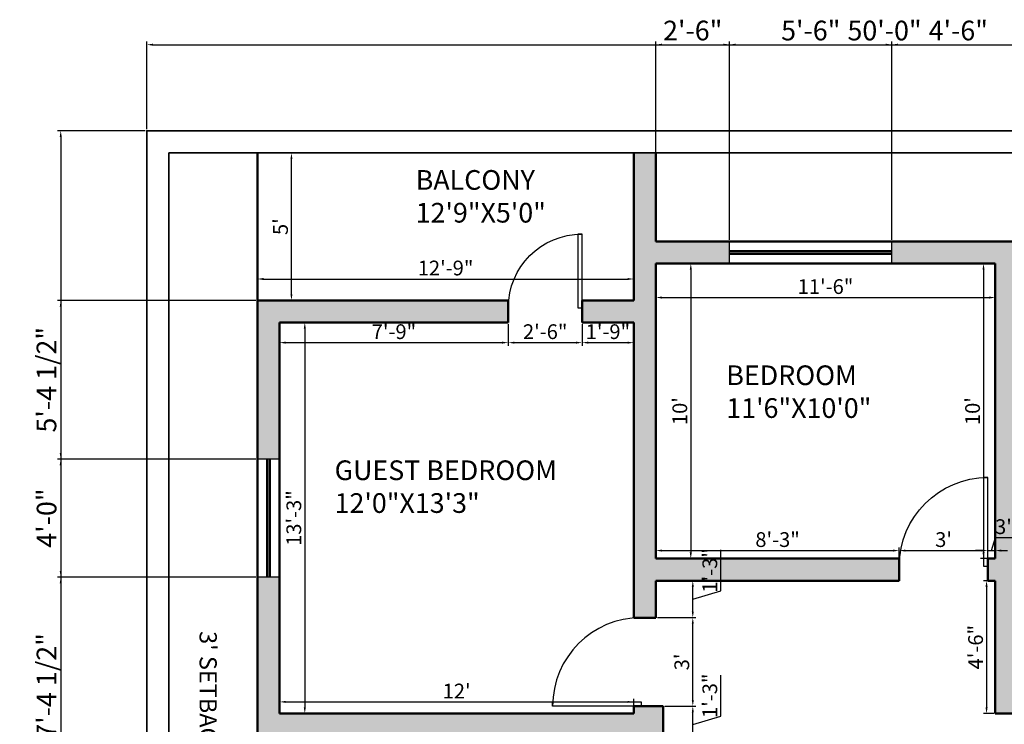
# Model space of a CAD drawing. Units: inches. Extents: x 2442 to 3851, y 589 to 2836.
# Tile 20 of 22: x 3157 to 3558, y 2550 to 2836. Entities that reach past the tile are written whole.
import ezdxf

# ---------------------------------------------------------------- set-up
doc = ezdxf.new("R2010")
doc.units = ezdxf.units.IN
for name, color, linetype, lineweight in [('A-ANNO-DIMS', 2, 'Continuous', 18), ('A-ANNO-TEXT', 7, 'Continuous', 18), ('A-AREA-IDEN', 7, 'Continuous', 18), ('A-DOOR', 4, 'Continuous', 25), ('A-GLAZ', 1, 'Continuous', 25), ('A-WALL', 7, 'Continuous', 50), ('A-WALL-PATT', 8, 'Continuous', 13), ('C-PROP', 7, 'Continuous', 35)]:
    doc.layers.add(name, color=color, linetype=linetype, lineweight=lineweight)
doc.styles.get("Standard").update_dxf_attribs({"font": 'arial.ttf'})
doc.dimstyles.new('ISO-25', dxfattribs={"dimtxt": 8, "dimasz": 2.5, "dimexe": 1.25, "dimexo": 0.625, "dimtad": 1, "dimlunit": 3, "dimtxsty": 'Standard', "dimcen": 2.5, "dimadec": 0, "dimazin": 0, "dimtfac": 1, "dimtmove": 0, "dimatfit": 3, "dimfxl": 1, "dimarcsym": 0})

# ---------------------------------------------------------------- blocks, each defined once
blk = doc.blocks.new('*U23')
for p, q in [((0, 0), (0, -6)), ((36, 0), (36, -6))]:
    blk.add_line(p, q)
blk.add_lwpolyline([(0, 0), (0, 36), (1.75, 36), (1.75, 0)], close=True)
blk.add_arc((0, 0), 36, 0, 90)
blk = doc.blocks.new('*U24')
for p, q in [((0, 0), (0, -6)), ((30, 0), (30, -6))]:
    blk.add_line(p, q)
blk.add_lwpolyline([(0, 0), (0, 30), (1.75, 30), (1.75, 0)], close=True)
blk.add_arc((0, 0), 30, 0, 90)
blk = doc.blocks.new('*D99')
at = {"layer": 'A-ANNO-DIMS', "color": 0, "lineweight": -2, "transparency": 16777216}
for p, q in [((3442.43, 2553.12), (3442.43, 2569.76)), ((3419.65, 2557.21), (3432.29, 2557.21)), ((3431.04, 2544.71), (3431.04, 2554.71)), ((3431.04, 2549.71), (3442.43, 2553.12)), ((3419.65, 2542.21), (3432.29, 2542.21))]:
    blk.add_line(p, q, dxfattribs=at)
at = {"layer": 'A-ANNO-DIMS', "color": 0, "transparency": 16777216}
for points in [[(3430.63, 2554.71), (3431.46, 2554.71), (3431.04, 2557.21)], [(3430.63, 2544.71), (3431.46, 2544.71), (3431.04, 2542.21)]]:
    blk.add_solid(points, dxfattribs=at)
at = {"layer": 'Defpoints', "color": 0, "transparency": 16777216}
for p in [(3419.02, 2557.21), (3431.04, 2557.21), (3419.02, 2542.21)]:
    blk.add_point(p, dxfattribs=at)
at = {"layer": 'A-ANNO-DIMS', "color": 0, "transparency": 16777216, "insert": (3438.74, 2561.44), "char_height": 6, "attachment_point": 5, "rotation": 90}
blk.add_mtext('1\'-3"', dxfattribs=at)
blk = doc.blocks.new('*D100')
at = {"layer": 'A-ANNO-DIMS', "color": 0, "lineweight": -2, "transparency": 16777216}
for p, q in [((3416.65, 2593.21), (3432.29, 2593.21)), ((3431.04, 2559.71), (3431.04, 2590.71)), ((3419.65, 2557.21), (3432.29, 2557.21))]:
    blk.add_line(p, q, dxfattribs=at)
at = {"layer": 'A-ANNO-DIMS', "color": 0, "transparency": 16777216}
for points in [[(3430.63, 2590.71), (3431.46, 2590.71), (3431.04, 2593.21)], [(3430.63, 2559.71), (3431.46, 2559.71), (3431.04, 2557.21)]]:
    blk.add_solid(points, dxfattribs=at)
at = {"layer": 'Defpoints', "color": 0, "transparency": 16777216}
for p in [(3416.02, 2593.21), (3431.04, 2593.21), (3419.02, 2557.21)]:
    blk.add_point(p, dxfattribs=at)
at = {"layer": 'A-ANNO-DIMS', "color": 0, "transparency": 16777216, "insert": (3427.35, 2575.21), "char_height": 6, "attachment_point": 5, "rotation": 90}
blk.add_mtext("3'", dxfattribs=at)
blk = doc.blocks.new('*D101')
at = {"layer": 'A-ANNO-DIMS', "color": 0, "lineweight": -2, "transparency": 16777216}
for p, q in [((3442.43, 2604.12), (3442.43, 2620.76)), ((3416.65, 2608.21), (3432.29, 2608.21)), ((3431.04, 2595.71), (3431.04, 2605.71)), ((3431.04, 2600.71), (3442.43, 2604.12)), ((3416.65, 2593.21), (3432.29, 2593.21))]:
    blk.add_line(p, q, dxfattribs=at)
at = {"layer": 'A-ANNO-DIMS', "color": 0, "transparency": 16777216}
for points in [[(3430.63, 2605.71), (3431.46, 2605.71), (3431.04, 2608.21)], [(3430.63, 2595.71), (3431.46, 2595.71), (3431.04, 2593.21)]]:
    blk.add_solid(points, dxfattribs=at)
at = {"layer": 'Defpoints', "color": 0, "transparency": 16777216}
for p in [(3416.02, 2608.21), (3431.04, 2608.21), (3416.02, 2593.21)]:
    blk.add_point(p, dxfattribs=at)
at = {"layer": 'A-ANNO-DIMS', "color": 0, "transparency": 16777216, "insert": (3438.74, 2612.44), "char_height": 6, "attachment_point": 5, "rotation": 90}
blk.add_mtext('1\'-3"', dxfattribs=at)
blk = doc.blocks.new('*D102')
at = {"layer": 'A-ANNO-DIMS', "color": 0, "lineweight": -2, "transparency": 16777216}
for p, q in [((3416.02, 2617.83), (3416.02, 2621.74)), ((3418.52, 2620.49), (3512.52, 2620.49)), ((3515.02, 2617.83), (3515.02, 2621.74))]:
    blk.add_line(p, q, dxfattribs=at)
at = {"layer": 'A-ANNO-DIMS', "color": 0, "transparency": 16777216}
for points in [[(3418.52, 2620.9), (3418.52, 2620.07), (3416.02, 2620.49)], [(3512.52, 2620.9), (3512.52, 2620.07), (3515.02, 2620.49)]]:
    blk.add_solid(points, dxfattribs=at)
at = {"layer": 'Defpoints', "color": 0, "transparency": 16777216}
for p in [(3515.02, 2620.49), (3416.02, 2617.21), (3515.02, 2617.21)]:
    blk.add_point(p, dxfattribs=at)
at = {"layer": 'A-ANNO-DIMS', "color": 0, "transparency": 16777216, "insert": (3465.52, 2624.18), "char_height": 6, "attachment_point": 5}
blk.add_mtext('8\'-3"', dxfattribs=at)
blk = doc.blocks.new('*D103')
at = {"layer": 'A-ANNO-DIMS', "color": 0, "lineweight": -2, "transparency": 16777216}
for p, q in [((3515.02, 2617.83), (3515.02, 2621.74)), ((3517.52, 2620.49), (3548.52, 2620.49)), ((3551.02, 2617.83), (3551.02, 2621.74))]:
    blk.add_line(p, q, dxfattribs=at)
at = {"layer": 'A-ANNO-DIMS', "color": 0, "transparency": 16777216}
for points in [[(3517.52, 2620.9), (3517.52, 2620.07), (3515.02, 2620.49)], [(3548.52, 2620.9), (3548.52, 2620.07), (3551.02, 2620.49)]]:
    blk.add_solid(points, dxfattribs=at)
at = {"layer": 'Defpoints', "color": 0, "transparency": 16777216}
for p in [(3551.02, 2620.49), (3515.02, 2617.21), (3551.02, 2617.21)]:
    blk.add_point(p, dxfattribs=at)
at = {"layer": 'A-ANNO-DIMS', "color": 0, "transparency": 16777216, "insert": (3533.02, 2624.18), "char_height": 6, "attachment_point": 5}
blk.add_mtext("3'", dxfattribs=at)
blk = doc.blocks.new('*D104')
at = {"layer": 'A-ANNO-DIMS', "color": 0, "lineweight": -2, "transparency": 16777216}
for p, q in [((3552.52, 2620.49), (3554.1, 2625.74)), ((3554.1, 2625.74), (3562.24, 2625.74)), ((3548.52, 2620.49), (3546.02, 2620.49)), ((3551.02, 2617.83), (3551.02, 2621.74)), ((3551.02, 2620.49), (3554.02, 2620.49)), ((3551.02, 2620.49), (3554.02, 2620.49)), ((3554.02, 2617.83), (3554.02, 2621.74)), ((3556.52, 2620.49), (3559.02, 2620.49))]:
    blk.add_line(p, q, dxfattribs=at)
at = {"layer": 'A-ANNO-DIMS', "color": 0, "transparency": 16777216}
for points in [[(3548.52, 2620.9), (3548.52, 2620.07), (3551.02, 2620.49)], [(3556.52, 2620.9), (3556.52, 2620.07), (3554.02, 2620.49)]]:
    blk.add_solid(points, dxfattribs=at)
at = {"layer": 'Defpoints', "color": 0, "transparency": 16777216}
for p in [(3554.02, 2620.49), (3551.02, 2617.21), (3554.02, 2617.21)]:
    blk.add_point(p, dxfattribs=at)
at = {"layer": 'A-ANNO-DIMS', "color": 0, "transparency": 16777216, "insert": (3558.17, 2629.43), "char_height": 6, "attachment_point": 5}
blk.add_mtext('3"', dxfattribs=at)
blk = doc.blocks.new('*D105')
at = {"layer": 'A-ANNO-DIMS', "color": 0, "lineweight": -2, "transparency": 16777216}
for p, q in [((3416.02, 2736.58), (3416.02, 2722.13)), ((3554.02, 2736.58), (3554.02, 2722.13)), ((3418.52, 2723.38), (3551.52, 2723.38))]:
    blk.add_line(p, q, dxfattribs=at)
at = {"layer": 'A-ANNO-DIMS', "color": 0, "transparency": 16777216}
for points in [[(3418.52, 2723.8), (3418.52, 2722.96), (3416.02, 2723.38)], [(3551.52, 2723.8), (3551.52, 2722.96), (3554.02, 2723.38)]]:
    blk.add_solid(points, dxfattribs=at)
at = {"layer": 'Defpoints', "color": 0, "transparency": 16777216}
for p in [(3416.02, 2737.21), (3554.02, 2737.21), (3554.02, 2723.38)]:
    blk.add_point(p, dxfattribs=at)
at = {"layer": 'A-ANNO-DIMS', "color": 0, "transparency": 16777216, "insert": (3485.02, 2727.07), "char_height": 6, "attachment_point": 5}
blk.add_mtext('11\'-6"', dxfattribs=at)
blk = doc.blocks.new('*D106')
at = {"layer": 'A-ANNO-DIMS', "color": 0, "lineweight": -2, "transparency": 16777216}
for p, q in [((3416.65, 2737.21), (3431.48, 2737.21)), ((3430.23, 2734.71), (3430.23, 2619.71)), ((3416.65, 2617.21), (3431.48, 2617.21))]:
    blk.add_line(p, q, dxfattribs=at)
at = {"layer": 'A-ANNO-DIMS', "color": 0, "transparency": 16777216}
for points in [[(3429.81, 2734.71), (3430.65, 2734.71), (3430.23, 2737.21)], [(3429.81, 2619.71), (3430.65, 2619.71), (3430.23, 2617.21)]]:
    blk.add_solid(points, dxfattribs=at)
at = {"layer": 'Defpoints', "color": 0, "transparency": 16777216}
for p in [(3416.02, 2737.21), (3416.02, 2617.21), (3430.23, 2617.21)]:
    blk.add_point(p, dxfattribs=at)
at = {"layer": 'A-ANNO-DIMS', "color": 0, "transparency": 16777216, "insert": (3426.54, 2677.21), "char_height": 6, "attachment_point": 5, "rotation": 90}
blk.add_mtext("10'", dxfattribs=at)
blk = doc.blocks.new('*D107')
at = {"layer": 'A-ANNO-DIMS', "color": 0, "lineweight": -2, "transparency": 16777216}
for p, q in [((3553.4, 2737.21), (3548.02, 2737.21)), ((3549.27, 2734.71), (3549.27, 2619.71)), ((3553.4, 2617.21), (3548.02, 2617.21))]:
    blk.add_line(p, q, dxfattribs=at)
at = {"layer": 'A-ANNO-DIMS', "color": 0, "transparency": 16777216}
for points in [[(3548.86, 2734.71), (3549.69, 2734.71), (3549.27, 2737.21)], [(3548.86, 2619.71), (3549.69, 2619.71), (3549.27, 2617.21)]]:
    blk.add_solid(points, dxfattribs=at)
at = {"layer": 'Defpoints', "color": 0, "transparency": 16777216}
for p in [(3554.02, 2737.21), (3549.27, 2617.21), (3554.02, 2617.21)]:
    blk.add_point(p, dxfattribs=at)
at = {"layer": 'A-ANNO-DIMS', "color": 0, "transparency": 16777216, "insert": (3545.59, 2677.21), "char_height": 6, "attachment_point": 5, "rotation": 90}
blk.add_mtext("10'", dxfattribs=at)
blk = doc.blocks.new('*D108')
at = {"layer": 'A-ANNO-DIMS', "color": 0, "lineweight": -2, "transparency": 16777216}
for p, q in [((3553.4, 2608.21), (3549.25, 2608.21)), ((3550.5, 2605.71), (3550.5, 2556.71)), ((3553.4, 2554.21), (3549.25, 2554.21))]:
    blk.add_line(p, q, dxfattribs=at)
at = {"layer": 'A-ANNO-DIMS', "color": 0, "transparency": 16777216}
for points in [[(3550.08, 2605.71), (3550.92, 2605.71), (3550.5, 2608.21)], [(3550.08, 2556.71), (3550.92, 2556.71), (3550.5, 2554.21)]]:
    blk.add_solid(points, dxfattribs=at)
at = {"layer": 'Defpoints', "color": 0, "transparency": 16777216}
for p in [(3554.02, 2608.21), (3550.5, 2554.21), (3554.02, 2554.21)]:
    blk.add_point(p, dxfattribs=at)
at = {"layer": 'A-ANNO-DIMS', "color": 0, "transparency": 16777216, "insert": (3546.81, 2581.21), "char_height": 6, "attachment_point": 5, "rotation": 90}
blk.add_mtext('4\'-6"', dxfattribs=at)
blk = doc.blocks.new('*D109')
at = {"layer": 'A-ANNO-DIMS', "color": 0, "lineweight": -2, "transparency": 16777216}
for p, q in [((3263.02, 2712.58), (3263.02, 2703.79)), ((3356.02, 2712.58), (3356.02, 2703.79)), ((3265.52, 2705.04), (3353.52, 2705.04))]:
    blk.add_line(p, q, dxfattribs=at)
at = {"layer": 'A-ANNO-DIMS', "color": 0, "transparency": 16777216}
for points in [[(3265.52, 2705.46), (3265.52, 2704.63), (3263.02, 2705.04)], [(3353.52, 2705.46), (3353.52, 2704.63), (3356.02, 2705.04)]]:
    blk.add_solid(points, dxfattribs=at)
at = {"layer": 'Defpoints', "color": 0, "transparency": 16777216}
for p in [(3263.02, 2713.21), (3356.02, 2713.21), (3356.02, 2705.04)]:
    blk.add_point(p, dxfattribs=at)
at = {"layer": 'A-ANNO-DIMS', "color": 0, "transparency": 16777216, "insert": (3309.52, 2708.73), "char_height": 6, "attachment_point": 5}
blk.add_mtext('7\'-9"', dxfattribs=at)
blk = doc.blocks.new('*D110')
at = {"layer": 'A-ANNO-DIMS', "color": 0, "lineweight": -2, "transparency": 16777216}
for p, q in [((3356.02, 2712.58), (3356.02, 2703.79)), ((3386.02, 2712.58), (3386.02, 2703.79)), ((3358.52, 2705.04), (3383.52, 2705.04))]:
    blk.add_line(p, q, dxfattribs=at)
at = {"layer": 'A-ANNO-DIMS', "color": 0, "transparency": 16777216}
for points in [[(3358.52, 2705.46), (3358.52, 2704.63), (3356.02, 2705.04)], [(3383.52, 2705.46), (3383.52, 2704.63), (3386.02, 2705.04)]]:
    blk.add_solid(points, dxfattribs=at)
at = {"layer": 'Defpoints', "color": 0, "transparency": 16777216}
for p in [(3356.02, 2713.21), (3386.02, 2713.21), (3386.02, 2705.04)]:
    blk.add_point(p, dxfattribs=at)
at = {"layer": 'A-ANNO-DIMS', "color": 0, "transparency": 16777216, "insert": (3371.02, 2708.73), "char_height": 6, "attachment_point": 5}
blk.add_mtext('2\'-6"', dxfattribs=at)
blk = doc.blocks.new('*D111')
at = {"layer": 'A-ANNO-DIMS', "color": 0, "lineweight": -2, "transparency": 16777216}
for p, q in [((3386.02, 2712.58), (3386.02, 2703.79)), ((3407.02, 2712.58), (3407.02, 2703.79)), ((3388.52, 2705.04), (3404.52, 2705.04))]:
    blk.add_line(p, q, dxfattribs=at)
at = {"layer": 'A-ANNO-DIMS', "color": 0, "transparency": 16777216}
for points in [[(3388.52, 2705.46), (3388.52, 2704.63), (3386.02, 2705.04)], [(3404.52, 2705.46), (3404.52, 2704.63), (3407.02, 2705.04)]]:
    blk.add_solid(points, dxfattribs=at)
at = {"layer": 'Defpoints', "color": 0, "transparency": 16777216}
for p in [(3386.02, 2713.21), (3407.02, 2713.21), (3407.02, 2705.04)]:
    blk.add_point(p, dxfattribs=at)
at = {"layer": 'A-ANNO-DIMS', "color": 0, "transparency": 16777216, "insert": (3396.52, 2708.73), "char_height": 6, "attachment_point": 5}
blk.add_mtext('1\'-9"', dxfattribs=at)
blk = doc.blocks.new('*D112')
at = {"layer": 'A-ANNO-DIMS', "color": 0, "lineweight": -2, "transparency": 16777216}
for p, q in [((3263.65, 2713.21), (3274.52, 2713.21)), ((3273.27, 2710.71), (3273.27, 2556.71)), ((3263.65, 2554.21), (3274.52, 2554.21))]:
    blk.add_line(p, q, dxfattribs=at)
at = {"layer": 'A-ANNO-DIMS', "color": 0, "transparency": 16777216}
for points in [[(3272.85, 2710.71), (3273.69, 2710.71), (3273.27, 2713.21)], [(3272.85, 2556.71), (3273.69, 2556.71), (3273.27, 2554.21)]]:
    blk.add_solid(points, dxfattribs=at)
at = {"layer": 'Defpoints', "color": 0, "transparency": 16777216}
for p in [(3263.02, 2713.21), (3263.02, 2554.21), (3273.27, 2554.21)]:
    blk.add_point(p, dxfattribs=at)
at = {"layer": 'A-ANNO-DIMS', "color": 0, "transparency": 16777216, "insert": (3269.58, 2633.71), "char_height": 6, "attachment_point": 5, "rotation": 90}
blk.add_mtext('13\'-3"', dxfattribs=at)
blk = doc.blocks.new('*D113')
at = {"layer": 'A-ANNO-DIMS', "color": 0, "lineweight": -2, "transparency": 16777216}
for p, q in [((3263.02, 2554.83), (3263.02, 2560.21)), ((3265.52, 2558.96), (3404.52, 2558.96)), ((3407.02, 2554.83), (3407.02, 2560.21))]:
    blk.add_line(p, q, dxfattribs=at)
at = {"layer": 'A-ANNO-DIMS', "color": 0, "transparency": 16777216}
for points in [[(3265.52, 2559.37), (3265.52, 2558.54), (3263.02, 2558.96)], [(3404.52, 2559.37), (3404.52, 2558.54), (3407.02, 2558.96)]]:
    blk.add_solid(points, dxfattribs=at)
at = {"layer": 'Defpoints', "color": 0, "transparency": 16777216}
for p in [(3407.02, 2558.96), (3263.02, 2554.21), (3407.02, 2554.21)]:
    blk.add_point(p, dxfattribs=at)
at = {"layer": 'A-ANNO-DIMS', "color": 0, "transparency": 16777216, "insert": (3335.02, 2562.59), "char_height": 6, "attachment_point": 5}
blk.add_mtext("12'", dxfattribs=at)
blk = doc.blocks.new('*D114')
at = {"layer": 'A-ANNO-DIMS', "color": 0, "lineweight": -2, "transparency": 16777216}
for p, q in [((3267.84, 2724.71), (3267.84, 2779.71)), ((3268.46, 2782.21), (3269.09, 2782.21)), ((3268.46, 2722.21), (3269.09, 2722.21))]:
    blk.add_line(p, q, dxfattribs=at)
at = {"layer": 'A-ANNO-DIMS', "color": 0, "transparency": 16777216}
for points in [[(3267.43, 2779.71), (3268.26, 2779.71), (3267.84, 2782.21)], [(3267.43, 2724.71), (3268.26, 2724.71), (3267.84, 2722.21)]]:
    blk.add_solid(points, dxfattribs=at)
at = {"layer": 'Defpoints', "color": 0, "transparency": 16777216}
for p in [(3267.84, 2782.21), (3267.84, 2782.21), (3267.84, 2722.21)]:
    blk.add_point(p, dxfattribs=at)
at = {"layer": 'A-ANNO-DIMS', "color": 0, "transparency": 16777216, "insert": (3264.17, 2752.21), "char_height": 6, "attachment_point": 5, "rotation": 90}
blk.add_mtext("5'", dxfattribs=at)
blk = doc.blocks.new('*D115')
at = {"layer": 'A-ANNO-DIMS', "color": 0, "lineweight": -2, "transparency": 16777216}
for p, q in [((3254.02, 2731.55), (3254.02, 2732.17)), ((3256.52, 2730.92), (3404.52, 2730.92)), ((3407.02, 2731.55), (3407.02, 2732.17))]:
    blk.add_line(p, q, dxfattribs=at)
at = {"layer": 'A-ANNO-DIMS', "color": 0, "transparency": 16777216}
for points in [[(3256.52, 2731.34), (3256.52, 2730.5), (3254.02, 2730.92)], [(3404.52, 2731.34), (3404.52, 2730.5), (3407.02, 2730.92)]]:
    blk.add_solid(points, dxfattribs=at)
at = {"layer": 'Defpoints', "color": 0, "transparency": 16777216}
for p in [(3254.02, 2730.92), (3407.02, 2730.92), (3407.02, 2730.92)]:
    blk.add_point(p, dxfattribs=at)
at = {"layer": 'A-ANNO-DIMS', "color": 0, "transparency": 16777216, "insert": (3330.52, 2734.61), "char_height": 6, "attachment_point": 5}
blk.add_mtext('12\'-9"', dxfattribs=at)
blk = doc.blocks.new('*D218')
at = {"layer": 'A-ANNO-DIMS', "color": 0, "lineweight": -2, "transparency": 16777216}
for p, q in [((3209.02, 2791.83), (3209.02, 2827.46)), ((3809.02, 2791.83), (3809.02, 2827.46)), ((3211.52, 2826.21), (3806.52, 2826.21))]:
    blk.add_line(p, q, dxfattribs=at)
at = {"layer": 'A-ANNO-DIMS', "color": 0, "transparency": 16777216}
for points in [[(3211.52, 2826.62), (3211.52, 2825.79), (3209.02, 2826.21)], [(3806.52, 2826.62), (3806.52, 2825.79), (3809.02, 2826.21)]]:
    blk.add_solid(points, dxfattribs=at)
at = {"layer": 'Defpoints', "color": 0, "transparency": 16777216}
for p in [(3809.02, 2826.21), (3209.02, 2791.21), (3809.02, 2791.21)]:
    blk.add_point(p, dxfattribs=at)
at = {"layer": 'A-ANNO-DIMS', "color": 0, "transparency": 16777216, "insert": (3509.02, 2830.92), "char_height": 8, "attachment_point": 5}
blk.add_mtext('50\'-0"', dxfattribs=at)
blk = doc.blocks.new('*D219')
at = {"layer": 'A-ANNO-DIMS', "color": 0, "lineweight": -2, "transparency": 16777216}
for p, q in [((3208.4, 2791.21), (3172.77, 2791.21)), ((3174.02, 2788.71), (3174.02, 2193.71)), ((3208.4, 2191.21), (3172.77, 2191.21))]:
    blk.add_line(p, q, dxfattribs=at)
at = {"layer": 'A-ANNO-DIMS', "color": 0, "transparency": 16777216}
for points in [[(3173.61, 2788.71), (3174.44, 2788.71), (3174.02, 2791.21)], [(3173.61, 2193.71), (3174.44, 2193.71), (3174.02, 2191.21)]]:
    blk.add_solid(points, dxfattribs=at)
at = {"layer": 'Defpoints', "color": 0, "transparency": 16777216}
for p in [(3209.02, 2791.21), (3174.02, 2191.21), (3209.02, 2191.21)]:
    blk.add_point(p, dxfattribs=at)
at = {"layer": 'A-ANNO-DIMS', "color": 0, "transparency": 16777216, "insert": (3169.31, 2491.21), "char_height": 8, "attachment_point": 5, "rotation": 90}
blk.add_mtext('50\'-0"', dxfattribs=at)
blk = doc.blocks.new('*D220')
at = {"layer": 'A-ANNO-DIMS', "color": 0, "lineweight": -2, "transparency": 16777216}
for p, q in [((3416.02, 2746.83), (3416.02, 2827.46)), ((3446.02, 2746.83), (3446.02, 2827.46)), ((3418.52, 2826.21), (3443.52, 2826.21))]:
    blk.add_line(p, q, dxfattribs=at)
at = {"layer": 'A-ANNO-DIMS', "color": 0, "transparency": 16777216}
for points in [[(3418.52, 2826.62), (3418.52, 2825.79), (3416.02, 2826.21)], [(3443.52, 2826.62), (3443.52, 2825.79), (3446.02, 2826.21)]]:
    blk.add_solid(points, dxfattribs=at)
at = {"layer": 'Defpoints', "color": 0, "transparency": 16777216}
for p in [(3446.02, 2826.21), (3416.02, 2746.21), (3446.02, 2746.21)]:
    blk.add_point(p, dxfattribs=at)
at = {"layer": 'A-ANNO-DIMS', "color": 0, "transparency": 16777216, "insert": (3431.02, 2830.92), "char_height": 8, "attachment_point": 5}
blk.add_mtext('2\'-6"', dxfattribs=at)
blk = doc.blocks.new('*D221')
at = {"layer": 'A-ANNO-DIMS', "color": 0, "lineweight": -2, "transparency": 16777216}
for p, q in [((3446.02, 2746.83), (3446.02, 2827.46)), ((3512.02, 2746.83), (3512.02, 2827.46)), ((3448.52, 2826.21), (3509.52, 2826.21))]:
    blk.add_line(p, q, dxfattribs=at)
at = {"layer": 'A-ANNO-DIMS', "color": 0, "transparency": 16777216}
for points in [[(3448.52, 2826.62), (3448.52, 2825.79), (3446.02, 2826.21)], [(3509.52, 2826.62), (3509.52, 2825.79), (3512.02, 2826.21)]]:
    blk.add_solid(points, dxfattribs=at)
at = {"layer": 'Defpoints', "color": 0, "transparency": 16777216}
for p in [(3512.02, 2826.21), (3446.02, 2746.21), (3512.02, 2746.21)]:
    blk.add_point(p, dxfattribs=at)
at = {"layer": 'A-ANNO-DIMS', "color": 0, "transparency": 16777216, "insert": (3479.02, 2830.92), "char_height": 8, "attachment_point": 5}
blk.add_mtext('5\'-6"', dxfattribs=at)
blk = doc.blocks.new('*D222')
at = {"layer": 'A-ANNO-DIMS', "color": 0, "lineweight": -2, "transparency": 16777216}
for p, q in [((3512.02, 2746.83), (3512.02, 2827.46)), ((3566.02, 2746.83), (3566.02, 2827.46)), ((3514.52, 2826.21), (3563.52, 2826.21))]:
    blk.add_line(p, q, dxfattribs=at)
at = {"layer": 'A-ANNO-DIMS', "color": 0, "transparency": 16777216}
for points in [[(3514.52, 2826.62), (3514.52, 2825.79), (3512.02, 2826.21)], [(3563.52, 2826.62), (3563.52, 2825.79), (3566.02, 2826.21)]]:
    blk.add_solid(points, dxfattribs=at)
at = {"layer": 'Defpoints', "color": 0, "transparency": 16777216}
for p in [(3566.02, 2826.21), (3512.02, 2746.21), (3566.02, 2746.21)]:
    blk.add_point(p, dxfattribs=at)
at = {"layer": 'A-ANNO-DIMS', "color": 0, "transparency": 16777216, "insert": (3539.02, 2830.92), "char_height": 8, "attachment_point": 5}
blk.add_mtext('4\'-6"', dxfattribs=at)
blk = doc.blocks.new('*D236')
at = {"layer": 'A-ANNO-DIMS', "color": 0, "lineweight": -2, "transparency": 16777216}
for p, q in [((3253.4, 2722.21), (3172.77, 2722.21)), ((3174.02, 2719.71), (3174.02, 2660.21)), ((3253.4, 2657.71), (3172.77, 2657.71))]:
    blk.add_line(p, q, dxfattribs=at)
at = {"layer": 'A-ANNO-DIMS', "color": 0, "transparency": 16777216}
for points in [[(3173.61, 2719.71), (3174.44, 2719.71), (3174.02, 2722.21)], [(3173.61, 2660.21), (3174.44, 2660.21), (3174.02, 2657.71)]]:
    blk.add_solid(points, dxfattribs=at)
at = {"layer": 'Defpoints', "color": 0, "transparency": 16777216}
for p in [(3254.02, 2722.21), (3174.02, 2657.71), (3254.02, 2657.71)]:
    blk.add_point(p, dxfattribs=at)
at = {"layer": 'A-ANNO-DIMS', "color": 0, "transparency": 16777216, "insert": (3169.26, 2689.96), "char_height": 8, "attachment_point": 5, "rotation": 90}
blk.add_mtext('5\'-4 1/2"', dxfattribs=at)
blk = doc.blocks.new('*D237')
at = {"layer": 'A-ANNO-DIMS', "color": 0, "lineweight": -2, "transparency": 16777216}
for p, q in [((3253.4, 2657.71), (3172.77, 2657.71)), ((3174.02, 2655.21), (3174.02, 2612.21)), ((3253.4, 2609.71), (3172.77, 2609.71))]:
    blk.add_line(p, q, dxfattribs=at)
at = {"layer": 'A-ANNO-DIMS', "color": 0, "transparency": 16777216}
for points in [[(3173.61, 2655.21), (3174.44, 2655.21), (3174.02, 2657.71)], [(3173.61, 2612.21), (3174.44, 2612.21), (3174.02, 2609.71)]]:
    blk.add_solid(points, dxfattribs=at)
at = {"layer": 'Defpoints', "color": 0, "transparency": 16777216}
for p in [(3254.02, 2657.71), (3174.02, 2609.71), (3254.02, 2609.71)]:
    blk.add_point(p, dxfattribs=at)
at = {"layer": 'A-ANNO-DIMS', "color": 0, "transparency": 16777216, "insert": (3169.31, 2633.71), "char_height": 8, "attachment_point": 5, "rotation": 90}
blk.add_mtext('4\'-0"', dxfattribs=at)
blk = doc.blocks.new('*D238')
at = {"layer": 'A-ANNO-DIMS', "color": 0, "lineweight": -2, "transparency": 16777216}
for p, q in [((3253.4, 2609.71), (3172.77, 2609.71)), ((3174.02, 2607.21), (3174.02, 2523.71)), ((3253.4, 2521.21), (3172.77, 2521.21))]:
    blk.add_line(p, q, dxfattribs=at)
at = {"layer": 'A-ANNO-DIMS', "color": 0, "transparency": 16777216}
for points in [[(3173.61, 2607.21), (3174.44, 2607.21), (3174.02, 2609.71)], [(3173.61, 2523.71), (3174.44, 2523.71), (3174.02, 2521.21)]]:
    blk.add_solid(points, dxfattribs=at)
at = {"layer": 'Defpoints', "color": 0, "transparency": 16777216}
for p in [(3254.02, 2609.71), (3174.02, 2521.21), (3254.02, 2521.21)]:
    blk.add_point(p, dxfattribs=at)
at = {"layer": 'A-ANNO-DIMS', "color": 0, "transparency": 16777216, "insert": (3169.26, 2565.46), "char_height": 8, "attachment_point": 5, "rotation": 90}
blk.add_mtext('7\'-4 1/2"', dxfattribs=at)

msp = doc.modelspace()

# ---------------------------------------------------------------- hatches: boundary and pattern name
at = {"layer": 'A-WALL-PATT'}
h = msp.add_hatch(color=256, dxfattribs=at)
h.dxf.hatch_style = 1
h.paths.add_polyline_path([(3356.024, 2713.208), (3356.024, 2719.208), (3356.024, 2722.208), (3254.024, 2722.208), (3254.024, 2657.708), (3263.024, 2657.708), (3263.024, 2713.208)])
h.paths.add_polyline_path([(3416.024, 2737.208), (3446.024, 2737.208), (3446.024, 2746.208), (3416.024, 2746.208), (3416.024, 2782.208), (3407.024, 2782.208), (3407.024, 2722.208), (3386.024, 2722.208), (3386.024, 2719.208), (3386.024, 2713.208), (3407.024, 2713.208), (3407.024, 2593.208), (3416.024, 2593.208), (3416.024, 2608.208), (3515.024, 2608.208), (3515.024, 2614.208), (3515.024, 2617.208), (3416.024, 2617.208)])
h.paths.add_polyline_path([(3563.024, 2737.208), (3566.024, 2737.208), (3566.024, 2746.208), (3512.024, 2746.208), (3512.024, 2737.208), (3554.024, 2737.208), (3554.024, 2617.208), (3551.024, 2617.208), (3551.024, 2614.208), (3551.024, 2608.208), (3554.024, 2608.208), (3554.024, 2554.208), (3566.024, 2554.208), (3566.024, 2560.208), (3566.024, 2563.208), (3563.024, 2563.208)])
h.paths.add_polyline_path([(3614.024, 2746.208), (3614.024, 2737.208), (3683.024, 2737.208), (3683.024, 2746.208)])
h.paths.add_polyline_path([(3755.024, 2737.208), (3755.024, 2665.208), (3764.024, 2665.208), (3764.024, 2746.208), (3731.024, 2746.208), (3731.024, 2737.208)])
h.paths.add_polyline_path([(3662.024, 2617.208), (3662.024, 2611.208), (3755.024, 2611.208), (3755.024, 2605.208), (3764.024, 2605.208), (3764.024, 2617.208)])
h.paths.add_polyline_path([(3755.024, 2554.208), (3755.024, 2548.208), (3764.024, 2548.208), (3764.024, 2569.208), (3755.024, 2569.208), (3755.024, 2563.208), (3677.024, 2563.208), (3677.024, 2581.208), (3671.024, 2581.208), (3671.024, 2563.208), (3611.024, 2563.208), (3611.024, 2611.208), (3632.024, 2611.208), (3632.024, 2617.208), (3605.024, 2617.208), (3605.024, 2563.208), (3602.024, 2563.208), (3602.024, 2554.208), (3653.024, 2554.208), (3653.024, 2536.208), (3659.024, 2536.208), (3659.024, 2554.208)])
h.paths.add_polyline_path([(3764.024, 2512.208), (3755.024, 2512.208), (3755.024, 2506.208), (3653.024, 2506.208), (3653.024, 2500.208), (3755.024, 2500.208), (3755.024, 2474.708), (3764.024, 2474.708)])
h.paths.add_polyline_path([(3608.024, 2392.208), (3764.024, 2392.208), (3764.024, 2426.708), (3755.024, 2426.708), (3755.024, 2401.208), (3608.024, 2401.208), (3608.024, 2461.208), (3599.024, 2461.208), (3599.024, 2353.208), (3608.024, 2353.208)])
h.paths.add_polyline_path([(3410.024, 2401.208), (3263.024, 2401.208), (3263.024, 2473.208), (3254.024, 2473.208), (3254.024, 2368.208), (3263.024, 2368.208), (3263.024, 2392.208), (3410.024, 2392.208), (3410.024, 2344.208), (3419.024, 2344.208), (3419.024, 2506.208), (3413.024, 2506.208), (3410.024, 2506.208)])
h.paths.add_polyline_path([(3263.024, 2609.708), (3254.024, 2609.708), (3254.024, 2521.208), (3263.024, 2521.208), (3263.024, 2545.208), (3410.024, 2545.208), (3410.024, 2542.208), (3413.024, 2542.208), (3419.024, 2542.208), (3419.024, 2557.208), (3407.024, 2557.208), (3407.024, 2554.208), (3263.024, 2554.208)])
h.paths.add_polyline_path([(3254.024, 2191.208), (3263.024, 2191.208), (3263.024, 2287.208), (3269.024, 2287.208), (3269.024, 2293.208), (3269.024, 2296.208), (3263.024, 2296.208), (3263.024, 2320.208), (3254.024, 2320.208)])
h.paths.add_polyline_path([(3419.024, 2296.208), (3386.024, 2296.208), (3386.024, 2287.208), (3410.024, 2287.208), (3410.024, 2191.208), (3419.024, 2191.208), (3419.024, 2248.208), (3449.024, 2248.208), (3449.024, 2257.208), (3419.024, 2257.208)])
h.paths.add_polyline_path([(3581.024, 2248.208), (3608.024, 2248.208), (3608.024, 2287.208), (3599.024, 2287.208), (3599.024, 2257.208), (3581.024, 2257.208)])
h.paths.add_polyline_path([(3491.024, 2248.208), (3515.024, 2248.208), (3515.024, 2257.208), (3491.024, 2257.208)])
h.paths.add_polyline_path([(3320.024, 2296.208), (3309.024, 2296.208), (3309.024, 2287.208), (3320.024, 2287.208)])
h.paths.add_polyline_path([(3282.007, 2631.263), (3387.059, 2631.263), (3387.059, 2661.678), (3282.007, 2661.678)], flags=9)
h.paths.add_polyline_path([(3511.253, 2214.916), (3571.545, 2214.916), (3571.545, 2229.862), (3511.253, 2229.862)], flags=9)
h.paths.add_polyline_path([(3777.335, 2589.915), (3777.335, 2529.623), (3792.281, 2529.623), (3792.281, 2589.915)], flags=9)
h.paths.add_polyline_path([(3558.97, 2754.629), (3619.262, 2754.629), (3619.262, 2769.575), (3558.97, 2769.575)], flags=9)
h.paths.add_polyline_path([(3314.979, 2749.318), (3377.263, 2749.318), (3377.263, 2779.733), (3314.979, 2779.733)], flags=9)
h.paths.add_polyline_path([(3624.453, 2577.252), (3671.045, 2577.252), (3671.045, 2600.063), (3624.453, 2600.063)], flags=25)
h.paths.add_polyline_path([(3701.15, 2577.252), (3744.07, 2577.252), (3744.07, 2600.063), (3701.15, 2600.063)], flags=25)
h.paths.add_polyline_path([(3689.533, 2518.545), (3731.868, 2518.545), (3731.868, 2541.356), (3689.533, 2541.356)], flags=9)
h.paths.add_polyline_path([(3629.196, 2666.979), (3693.452, 2666.979), (3693.452, 2697.394), (3629.196, 2697.394)], flags=9)
h.paths.add_polyline_path([(3441.284, 2669.891), (3505.54, 2669.891), (3505.54, 2700.306), (3441.284, 2700.306)], flags=25)
h.paths.add_polyline_path([(3306.565, 2459.233), (3370.821, 2459.233), (3370.821, 2489.648), (3306.565, 2489.648)], flags=25)
h.paths.add_polyline_path([(3307.889, 2320.733), (3387.355, 2320.733), (3387.355, 2351.148), (3307.889, 2351.148)], flags=9)
h.paths.add_polyline_path([(3452.987, 2372.794), (3554.971, 2372.794), (3554.971, 2403.208), (3452.987, 2403.208)], flags=9)

# ---------------------------------------------------------------- linework, layer by layer
at = {"layer": 'A-GLAZ'}
for p, q in [((3446.024, 2737.208), (3446.024, 2746.208)), ((3512.024, 2737.208), (3512.024, 2746.208)), ((3263.024, 2657.708), (3254.024, 2657.708)), ((3263.024, 2609.708), (3254.024, 2609.708))]:
    msp.add_line(p, q, dxfattribs=at)
at = {"layer": 'A-WALL'}
for p, q in [((3254.024, 2782.208), (3254.024, 2191.208)), ((3407.024, 2722.208), (3407.024, 2782.208)), ((3416.024, 2746.208), (3416.024, 2782.208)), ((3416.024, 2746.208), (3764.024, 2746.208)), ((3446.024, 2742.208), (3512.024, 2742.208)), ((3446.024, 2741.208), (3512.024, 2741.208)), ((3416.024, 2617.208), (3416.024, 2737.208)), ((3416.024, 2737.208), (3554.024, 2737.208)), ((3554.024, 2617.208), (3554.024, 2737.208)), ((3254.024, 2722.208), (3356.024, 2722.208)), ((3356.024, 2713.208), (3356.024, 2722.208)), ((3386.024, 2713.208), (3386.024, 2722.208)), ((3386.024, 2722.208), (3407.024, 2722.208)), ((3263.024, 2713.208), (3263.024, 2554.208)), ((3263.024, 2713.208), (3356.024, 2713.208)), ((3386.024, 2713.208), (3407.024, 2713.208)), ((3407.024, 2593.208), (3407.024, 2713.208)), ((3258.024, 2657.708), (3258.024, 2609.708)), ((3259.024, 2657.708), (3259.024, 2609.708)), ((3416.024, 2617.208), (3515.024, 2617.208)), ((3515.024, 2608.208), (3515.024, 2617.208)), ((3551.024, 2608.208), (3551.024, 2617.208)), ((3551.024, 2617.208), (3554.024, 2617.208)), ((3416.024, 2593.208), (3416.024, 2608.208)), ((3416.024, 2608.208), (3515.024, 2608.208)), ((3551.024, 2608.208), (3554.024, 2608.208)), ((3554.024, 2554.208), (3554.024, 2608.208)), ((3407.024, 2593.208), (3416.024, 2593.208)), ((3407.024, 2554.208), (3407.024, 2557.208)), ((3407.024, 2557.208), (3419.024, 2557.208)), ((3419.024, 2542.208), (3419.024, 2557.208)), ((3263.024, 2554.208), (3407.024, 2554.208)), ((3554.024, 2554.208), (3566.024, 2554.208))]:
    msp.add_line(p, q, dxfattribs=at)
at = {"layer": 'C-PROP'}
for points in [[(3809.024, 2191.208), (3809.024, 2791.208), (3209.024, 2791.208), (3209.024, 2191.208), (3809.024, 2191.208)], [(3800.024, 2200.208), (3800.024, 2782.208), (3218.024, 2782.208), (3218.024, 2200.208), (3254.024, 2200.208)]]:
    msp.add_lwpolyline(points, dxfattribs=at)

# ---------------------------------------------------------------- block references
at = {"layer": 'A-DOOR', "xscale": -1}
for name, p in [('*U24', (3386.024, 2719.208)), ('*U23', (3551.024, 2614.208))]:
    msp.add_blockref(name, p, dxfattribs=at)
at = {"layer": 'A-DOOR', "rotation": 90.00000000000003}
msp.add_blockref('*U23', (3410.024, 2557.208), dxfattribs=at)

# ---------------------------------------------------------------- texts
at = {"layer": 'A-ANNO-TEXT', "insert": (3237.481, 2587.746), "char_height": 7, "attachment_point": 1, "rotation": 270}
msp.add_mtext_dynamic_manual_height_columns("{\\fTimes New Roman|b0|i0|c0|p18;3' SETBACK}", width=79.56037, gutter_width=12.5, heights=[0], dxfattribs=at)
at = {"layer": 'A-AREA-IDEN', "char_height": 8, "attachment_point": 1}
for s, insert in [('{\\fTimes New Roman|b0|i0|c0|p18;BALCONY\\P12\'9"X5\'0"}', (3318.363, 2775.206)), ('{\\fTimes New Roman|b0|i0|c0|p18;BEDROOM\\P11\'6"X10\'0"}', (3444.668, 2695.78)), ('{\\fTimes New Roman|b0|i0|c0|p18;GUEST BEDROOM\\P12\'0"X13\'3"}', (3285.391, 2657.152))]:
    msp.add_mtext_dynamic_manual_height_columns(s, width=110.76054, gutter_width=12.5, heights=[0], dxfattribs=dict(at, insert=insert))

# ---------------------------------------------------------------- dimensions: what is measured, and where the dimension line sits
at = {"layer": 'A-ANNO-DIMS'}
for base, p1, p2, override, picture, middle in [((3809.024, 2826.208), (3209.024, 2791.208), (3809.024, 2791.208), {"dimdec": 1, "dimlfac": 1, "dimrnd": 0, "dimzin": 1, "dimdsep": 46, "dimlunit": 4, "dimfrac": 2}, '*D218', (3509.024, 2830.917)), ((3446.024, 2826.208), (3416.024, 2746.208), (3446.024, 2746.208), {"dimdec": 1, "dimlfac": 1, "dimrnd": 0, "dimzin": 1, "dimdsep": 46, "dimlunit": 4, "dimfrac": 2}, '*D220', (3431.024, 2830.917)), ((3512.024, 2826.208), (3446.024, 2746.208), (3512.024, 2746.208), {"dimdec": 1, "dimlfac": 1, "dimrnd": 0, "dimzin": 1, "dimdsep": 46, "dimlunit": 4, "dimfrac": 2}, '*D221', (3479.024, 2830.917)), ((3566.024, 2826.208), (3512.024, 2746.208), (3566.024, 2746.208), {"dimdec": 1, "dimlfac": 1, "dimrnd": 0, "dimzin": 1, "dimdsep": 46, "dimlunit": 4, "dimfrac": 2}, '*D222', (3539.024, 2830.917)), ((3407.024, 2730.921), (3254.024, 2730.921), (3407.024, 2730.921), {"dimtxt": 6, "dimclrd": 0, "dimclre": 0, "dimclrt": 0}, '*D115', (3330.524, 2734.609)), ((3554.024, 2723.381), (3416.024, 2737.208), (3554.024, 2737.208), {"dimtxt": 6, "dimclrd": 0, "dimclre": 0, "dimclrt": 0}, '*D105', (3485.024, 2727.07)), ((3356.024, 2705.042), (3263.024, 2713.208), (3356.024, 2713.208), {"dimtxt": 6, "dimclrd": 0, "dimclre": 0, "dimclrt": 0}, '*D109', (3309.524, 2708.731)), ((3386.024, 2705.042), (3356.024, 2713.208), (3386.024, 2713.208), {"dimtxt": 6, "dimclrd": 0, "dimclre": 0, "dimclrt": 0, "dimtmove": 1}, '*D110', (3371.024, 2708.731)), ((3407.024, 2705.042), (3386.024, 2713.208), (3407.024, 2713.208), {"dimtxt": 6, "dimclrd": 0, "dimclre": 0, "dimclrt": 0, "dimtmove": 1}, '*D111', (3396.524, 2708.731)), ((3554.024, 2620.486), (3551.024, 2617.208), (3554.024, 2617.208), {"dimtxt": 6, "dimclrd": 0, "dimclre": 0, "dimclrt": 0, "dimtmove": 1}, '*D104', (3554.725, 2629.429)), ((3515.024, 2620.486), (3416.024, 2617.208), (3515.024, 2617.208), {"dimtxt": 6, "dimclrd": 0, "dimclre": 0, "dimclrt": 0}, '*D102', (3465.524, 2624.176)), ((3551.024, 2620.486), (3515.024, 2617.208), (3551.024, 2617.208), {"dimtxt": 6, "dimclrd": 0, "dimclre": 0, "dimclrt": 0, "dimtmove": 1}, '*D103', (3533.024, 2624.176)), ((3407.024, 2558.958), (3263.024, 2554.208), (3407.024, 2554.208), {"dimtxt": 6, "dimclrd": 0, "dimclre": 0, "dimclrt": 0}, '*D113', (3335.024, 2562.595))]:
    dim = msp.add_linear_dim(base=base, p1=p1, p2=p2, dimstyle='ISO-25', override=override, dxfattribs=at)
    dim.commit()
    dim.dimension.update_dxf_attribs({"geometry": picture, "text_midpoint": middle})
for base, p1, p2, override, picture, middle in [((3174.024, 2191.208), (3209.024, 2791.208), (3209.024, 2191.208), {"dimdec": 1, "dimlfac": 1, "dimrnd": 0, "dimzin": 1, "dimdsep": 46, "dimlunit": 4, "dimfrac": 2}, '*D219', (3169.315, 2491.208)), ((3267.842, 2782.208), (3267.838, 2722.208), (3267.838, 2782.208), {"dimtxt": 6, "dimclrd": 0, "dimclre": 0, "dimclrt": 0}, '*D114', (3264.166, 2752.208)), ((3430.229, 2617.208), (3416.024, 2737.208), (3416.024, 2617.208), {"dimtxt": 6, "dimclrd": 0, "dimclre": 0, "dimclrt": 0}, '*D106', (3426.54, 2677.208)), ((3549.274, 2617.208), (3554.024, 2737.208), (3554.024, 2617.208), {"dimtxt": 6, "dimclrd": 0, "dimclre": 0, "dimclrt": 0}, '*D107', (3545.586, 2677.208)), ((3174.024, 2657.708), (3254.024, 2722.208), (3254.024, 2657.708), {"dimdec": 1, "dimlfac": 1, "dimrnd": 0, "dimzin": 1, "dimdsep": 46, "dimlunit": 4, "dimfrac": 2}, '*D236', (3169.263, 2689.958)), ((3273.268, 2554.208), (3263.024, 2713.208), (3263.024, 2554.208), {"dimtxt": 6, "dimclrd": 0, "dimclre": 0, "dimclrt": 0}, '*D112', (3269.578, 2633.708)), ((3174.024, 2609.708), (3254.024, 2657.708), (3254.024, 2609.708), {"dimdec": 1, "dimlfac": 1, "dimrnd": 0, "dimzin": 1, "dimdsep": 46, "dimlunit": 4, "dimfrac": 2}, '*D237', (3169.315, 2633.708)), ((3431.044, 2608.208), (3416.024, 2593.208), (3416.024, 2608.208), {"dimtxt": 6, "dimclrd": 0, "dimclre": 0, "dimclrt": 0, "dimtmove": 1}, '*D101', (3438.737, 2604.748)), ((3174.024, 2521.208), (3254.024, 2609.708), (3254.024, 2521.208), {"dimdec": 1, "dimlfac": 1, "dimrnd": 0, "dimzin": 1, "dimdsep": 46, "dimlunit": 4, "dimfrac": 2}, '*D238', (3169.263, 2565.458)), ((3550.499, 2554.208), (3554.024, 2608.208), (3554.024, 2554.208), {"dimtxt": 6, "dimclrd": 0, "dimclre": 0, "dimclrt": 0}, '*D108', (3546.811, 2581.208)), ((3431.044, 2593.208), (3419.024, 2557.208), (3416.024, 2593.208), {"dimtxt": 6, "dimclrd": 0, "dimclre": 0, "dimclrt": 0, "dimtmove": 1}, '*D100', (3427.353, 2575.208)), ((3431.044, 2557.208), (3419.024, 2542.208), (3419.024, 2557.208), {"dimtxt": 6, "dimclrd": 0, "dimclre": 0, "dimclrt": 0, "dimtmove": 1}, '*D99', (3438.737, 2553.748))]:
    dim = msp.add_linear_dim(base=base, p1=p1, p2=p2, angle=90, dimstyle='ISO-25', override=override, dxfattribs=at)
    dim.commit()
    dim.dimension.update_dxf_attribs({"geometry": picture, "text_midpoint": middle})

doc.saveas('drawing.dxf')
